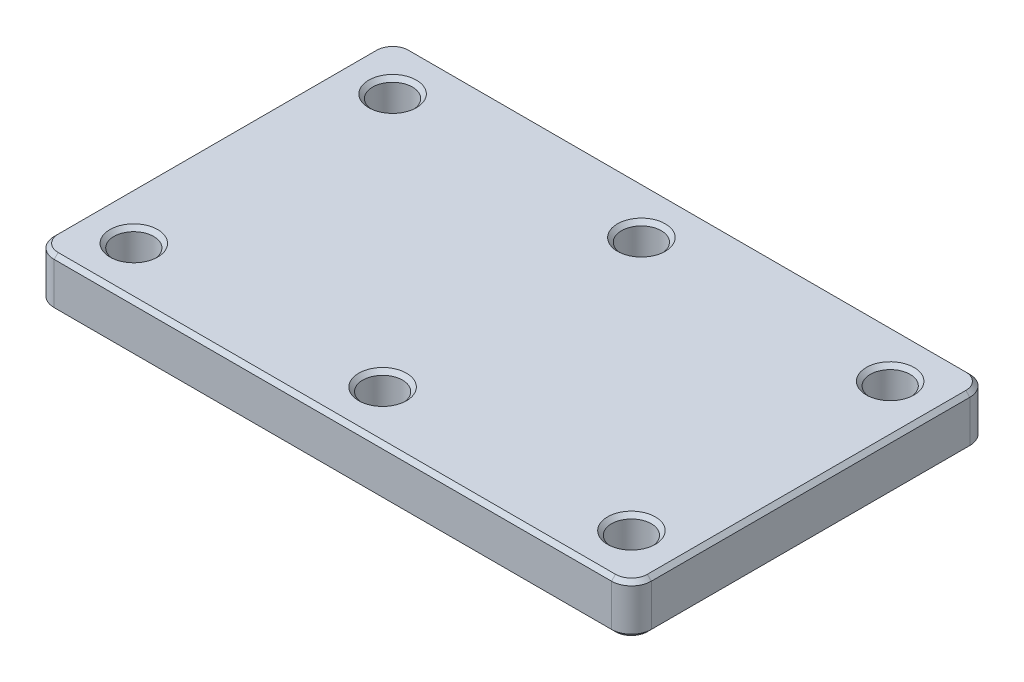
from build123d import *

# Parameters (mm, degrees)
PLATE_OUTLINE_AND_HOLE_SKETCH_R = 10
BASE_PLATE_25MM_DEPTH           = 25
EDGE_CHAMFER_2X45DEG_SIZE       = 2


with BuildPart() as part:
    # Plate Outline and Hole Sketch → Base Plate 25mm (new body)
    with BuildSketch(Plane(origin=(0, 0, 0), x_dir=(1, 0, 0), z_dir=(0, 1, 0))):
        with BuildLine():
            Line((-140, 90), (140, 90))
            ThreePointArc((140, 90), (147.071067812, 87.071067812), (150, 80))
            Line((150, 80), (150, -80))
            ThreePointArc((150, -80), (147.071067812, -87.071067812), (140, -90))
            Line((140, -90), (-140, -90))
            ThreePointArc((-140, -90), (-147.071067812, -87.071067812), (-150, -80))
            Line((-150, -80), (-150, 80))
            ThreePointArc((-150, 80), (-147.071067812, 87.071067812), (-140, 90))
        make_face()
        with Locations(Location((-125, 65, 0), (0, 0, 270))):
            Circle(PLATE_OUTLINE_AND_HOLE_SKETCH_R, mode=Mode.SUBTRACT)
        with Locations(Location((-125, -65, 0), (0, 0, 90))):
            Circle(PLATE_OUTLINE_AND_HOLE_SKETCH_R, mode=Mode.SUBTRACT)
        with Locations(Location((125, 65, 0), (0, 0, 90))):
            Circle(PLATE_OUTLINE_AND_HOLE_SKETCH_R, mode=Mode.SUBTRACT)
        with Locations(Location((125, -65, 0), (0, 0, 270))):
            Circle(PLATE_OUTLINE_AND_HOLE_SKETCH_R, mode=Mode.SUBTRACT)
        with Locations(Location((0, 65, 0), (0, 0, 270))):
            Circle(PLATE_OUTLINE_AND_HOLE_SKETCH_R, mode=Mode.SUBTRACT)
        with Locations(Location((0, -65, 0), (0, 0, 270))):
            Circle(PLATE_OUTLINE_AND_HOLE_SKETCH_R, mode=Mode.SUBTRACT)
    extrude(amount=BASE_PLATE_25MM_DEPTH)

    # Edge Chamfer 2x45deg
    edge_chamfer_2x45deg_edges = [part.edges().sort_by_distance(p)[0] for p in [
        (-150, 0, 0),
        (-147.071067812, 0, -87.071067812),
        (0, 0, -90),
        (147.071067812, 0, -87.071067812),
        (-147.071067812, 25, -87.071067812),
        (-150, 25, 0),
        (-147.071067812, 25, 87.071067812),
        (-125, 0, -75),
        (-125, 25, -75),
        (0, 25, 90),
        (-125, 0, 75),
        (-125, 25, 75),
        (147.071067812, 25, 87.071067812),
        (125, 0, -55),
        (125, 25, -55),
        (150, 25, 0),
        (125, 0, 55),
        (125, 25, 55),
        (0, 0, -75),
        (0, 25, -75),
        (0, 0, 55),
        (0, 25, 55),
        (147.071067812, 25, -87.071067812),
        (150, 0, 0),
        (0, 25, -90),
        (147.071067812, 0, 87.071067812),
        (0, 0, 90),
        (-147.071067812, 0, 87.071067812),
    ]]
    chamfer(edge_chamfer_2x45deg_edges, length=EDGE_CHAMFER_2X45DEG_SIZE)


solid = part.part
